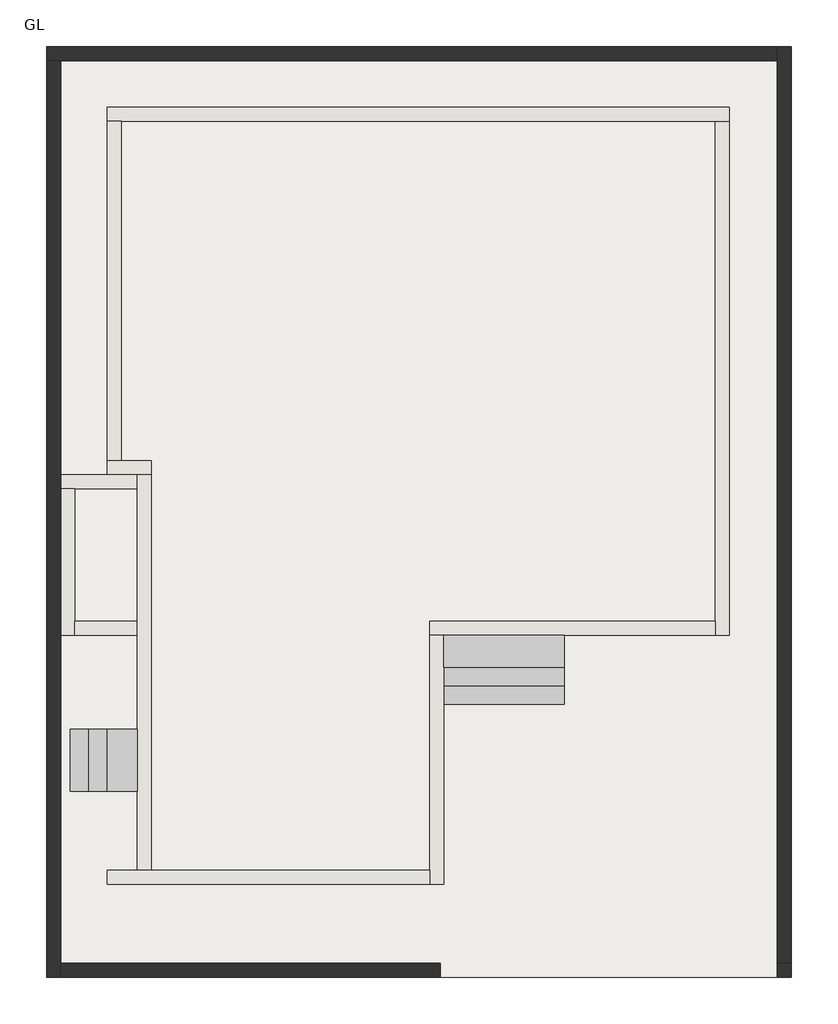
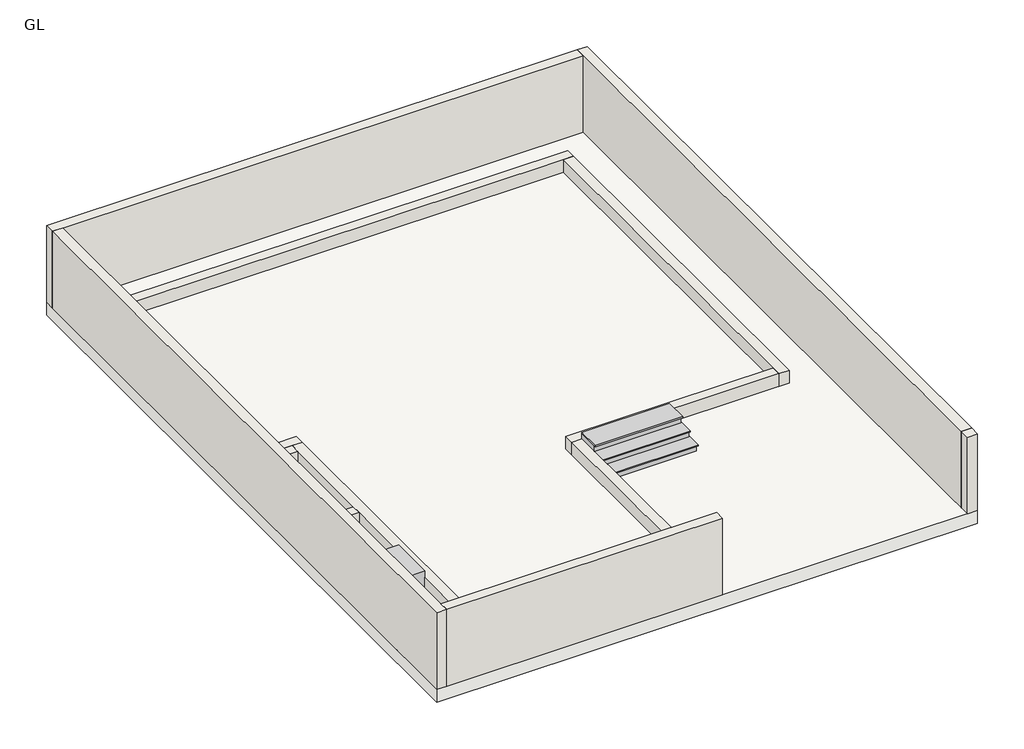
# One storey: 15 walls, 2 proxies, 1 slab.
"""IFC4 building model written with IfcOpenShell, lengths in millimetres."""

from ifc_helpers import new_model, si_unit, frame, origin, place, context, project, spatial, polyline, outline, extrude, faceted_brep, transform, mapped, element, save
from components import generic_models_1_generic_models_1_70b2dbcb, generic_models_2_generic_models_1_31704990

model = new_model("IFC4")

# Units and contexts
model_context = context("Model", 3, world=origin())
ifc_project = project(units=[si_unit("LENGTHUNIT", "METRE", prefix="MILLI")], contexts=[model_context])

# Site, building, storey
site = spatial("IfcSite", under=ifc_project)
building = spatial("IfcBuilding", under=site)
storey = spatial("IfcBuildingStorey", under=building, Name="GL", Elevation=-457.2)

# Proxies
placement = place(None, origin())
generic_models_1_generic_models_1_shape = generic_models_1_generic_models_1_70b2dbcb(model_context)
element("IfcBuildingElementProxy", 1, Name="Generic Models 1 : Generic Models 1", ObjectType="Generic Models 1 : Generic Models 1", at=placement, inside=storey, context=model_context, shape_type="MappedRepresentation", body=[
    mapped(generic_models_1_generic_models_1_shape, transform((0.0, 0.0, 0.0), x_axis=(1.0, 0.0, 0.0), y_axis=(0.0, 1.0, 0.0), z_axis=(0.0, 0.0, 1.0))),
])
generic_models_2_generic_models_1_shape = generic_models_2_generic_models_1_31704990(model_context)
element("IfcBuildingElementProxy", 2, Name="Generic Models 2 : Generic Models 1", ObjectType="Generic Models 2 : Generic Models 1", at=placement, inside=storey, context=model_context, shape_type="MappedRepresentation", body=[
    mapped(generic_models_2_generic_models_1_shape, transform((-17182.3129808, -6192.8854878, 0.0), x_axis=(0.0, -1.0, 0.0), y_axis=(1.0, 0.0, 0.0), z_axis=(0.0, 0.0, 1.0))),
])

# Slab
element("IfcSlab", 3, ObjectType="Generic - 12\"", at=placement, inside=storey, context=model_context, shape_type="SweptSolid", body=[
    extrude(outline(polyline([(-2722.9002526, 13392.6128362), (-2722.9002526, -1847.3871638), (-14917.2815026, -1847.3871638), (-14917.2815026, 13392.6128362), (-2722.9002526, 13392.6128362)])), frame((0.0, 0.0, -762.0), z_axis=(0.0, 0.0, 1.0), x_axis=(1.0, 0.0, 0.0)), (0.0, 0.0, 1.0), 304.8),
])

# Walls
element("IfcWall", 4, ObjectType="10\"", at=placement, inside=storey, context=model_context, shape_type="Brep", body=[
    faceted_brep([(-13924.3002526, 12173.4128362, -457.2), (-13695.7002526, 12173.4128362, -457.2), (-3967.5002526, 12173.4128362, -457.2), (-3738.9002526, 12173.4128362, -457.2), (-3738.9002526, 12173.4128362, -152.4), (-3967.5002526, 12173.4128362, -152.4), (-13695.7002526, 12173.4128362, -152.4), (-13924.3002526, 12173.4128362, -152.4), (-13924.3002526, 12402.0128362, -457.2), (-13924.3002526, 12402.0128362, -152.4), (-3738.9002526, 12402.0128362, -152.4), (-3738.9002526, 12402.0128362, -457.2)], [[[0, 1, 2, 3, 4, 5, 6, 7]], [[8, 9, 10, 11]], [[3, 2, 1, 0, 8, 11]], [[7, 6, 5, 4, 10, 9]], [[0, 7, 9, 8]], [[4, 3, 11, 10]]]),
])
element("IfcWall", 5, ObjectType="10\"", at=placement, inside=storey, context=model_context, shape_type="SweptSolid", body=[
    extrude(outline(polyline([(-13695.7002526, 12173.4128362), (-13695.7002526, 6610.8128362), (-13924.3002526, 6610.8128362), (-13924.3002526, 12173.4128362), (-13695.7002526, 12173.4128362)])), frame((0.0, 0.0, -457.2), z_axis=(0.0, 0.0, 1.0), x_axis=(1.0, 0.0, 0.0)), (0.0, 0.0, 1.0), 304.8),
])
element("IfcWall", 6, ObjectType="10\"", at=placement, inside=storey, context=model_context, shape_type="Brep", body=[
    faceted_brep([(-3967.5002526, 12173.4128362, -457.2), (-3967.5002526, 3981.9127283, -457.2), (-3967.5002526, 3753.3127283, -457.2), (-3967.5002526, 3753.3127283, -152.4), (-3967.5002526, 3981.9127283, -152.4), (-3967.5002526, 12173.4128362, -152.4), (-3738.9002526, 12173.4128362, -457.2), (-3738.9002526, 12173.4128362, -152.4), (-3738.9002526, 3753.3127283, -152.4), (-3738.9002526, 3753.3127283, -457.2)], [[[0, 1, 2, 3, 4, 5]], [[6, 7, 8, 9]], [[2, 1, 0, 6, 9]], [[5, 4, 3, 8, 7]], [[0, 5, 7, 6]], [[3, 2, 9, 8]]]),
])
element("IfcWall", 7, ObjectType="10\"", at=placement, inside=storey, context=model_context, shape_type="Brep", body=[
    faceted_brep([(-3967.5002526, 3981.9127283, -457.2), (-8641.1002526, 3981.9127283, -457.2), (-8641.1002526, 3981.9127283, -152.4), (-3967.5002526, 3981.9127283, -152.4), (-3967.5002526, 3753.3127283, -457.2), (-3967.5002526, 3753.3127283, -152.4), (-8412.5002526, 3753.3127283, -152.4), (-8641.1002526, 3753.3127283, -152.4), (-8641.1002526, 3753.3127283, -457.2), (-8412.5002526, 3753.3127283, -457.2)], [[[0, 1, 2, 3]], [[4, 5, 6, 7, 8, 9]], [[1, 0, 4, 9, 8]], [[3, 2, 7, 6, 5]], [[0, 3, 5, 4]], [[2, 1, 8, 7]]]),
])
element("IfcWall", 8, ObjectType="10\"", at=placement, inside=storey, context=model_context, shape_type="Brep", body=[
    faceted_brep([(-8641.1002526, 3753.3127283, -457.2), (-8641.1002526, -92.4059138, -457.2), (-8641.1002526, -321.0059138, -457.2), (-8641.1002526, -321.0059138, -152.4), (-8641.1002526, -92.4059138, -152.4), (-8641.1002526, 3753.3127283, -152.4), (-8412.5002526, 3753.3127283, -457.2), (-8412.5002526, 3753.3127283, -152.4), (-8412.5002526, -321.0059138, -152.4), (-8412.5002526, -321.0059138, -457.2)], [[[0, 1, 2, 3, 4, 5]], [[6, 7, 8, 9]], [[2, 1, 0, 6, 9]], [[5, 4, 3, 8, 7]], [[0, 5, 7, 6]], [[3, 2, 9, 8]]]),
])
element("IfcWall", 9, ObjectType="10\"", at=placement, inside=storey, context=model_context, shape_type="Brep", body=[
    faceted_brep([(-8641.1002526, -92.4059138, -457.2), (-13200.4002526, -92.4059138, -457.2), (-13429.0002526, -92.4059138, -457.2), (-13925.8877526, -92.4059138, -457.2), (-13925.8877526, -92.4059138, -152.4), (-13429.0002526, -92.4059138, -152.4), (-13200.4002526, -92.4059138, -152.4), (-8641.1002526, -92.4059138, -152.4), (-8641.1002526, -321.0059138, -457.2), (-8641.1002526, -321.0059138, -152.4), (-13925.8877526, -321.0059138, -152.4), (-13925.8877526, -321.0059138, -457.2)], [[[0, 1, 2, 3, 4, 5, 6, 7]], [[8, 9, 10, 11]], [[3, 2, 1, 0, 8, 11]], [[4, 3, 11, 10]], [[7, 6, 5, 4, 10, 9]], [[0, 7, 9, 8]]]),
])
element("IfcWall", 10, ObjectType="10\"", at=placement, inside=storey, context=model_context, shape_type="Brep", body=[
    faceted_brep([(-13200.4002526, -92.4059138, -457.2), (-13200.4002526, 6382.2128362, -457.2), (-13200.4002526, 6382.2128362, -152.4), (-13200.4002526, -92.4059138, -152.4), (-13429.0002526, -92.4059138, -457.2), (-13429.0002526, -92.4059138, -152.4), (-13429.0002526, 3752.3673766, -152.4), (-13429.0002526, 3980.9673766, -152.4), (-13429.0002526, 6153.6128362, -152.4), (-13429.0002526, 6382.2128362, -152.4), (-13429.0002526, 6382.2128362, -457.2), (-13429.0002526, 6153.6128362, -457.2), (-13429.0002526, 3980.9673766, -457.2), (-13429.0002526, 3752.3673766, -457.2)], [[[0, 1, 2, 3]], [[4, 5, 6, 7, 8, 9, 10, 11, 12, 13]], [[1, 0, 4, 13, 12, 11, 10]], [[3, 2, 9, 8, 7, 6, 5]], [[0, 3, 5, 4]], [[2, 1, 10, 9]]]),
])
element("IfcWall", 11, ObjectType="10\"", at=placement, inside=storey, context=model_context, shape_type="Brep", body=[
    faceted_brep([(-13924.3002526, 6382.2128362, -457.2), (-13429.0002526, 6382.2128362, -457.2), (-13200.4002526, 6382.2128362, -457.2), (-13200.4002526, 6382.2128362, -152.4), (-13429.0002526, 6382.2128362, -152.4), (-13924.3002526, 6382.2128362, -152.4), (-13924.3002526, 6610.8128362, -457.2), (-13924.3002526, 6610.8128362, -152.4), (-13695.7002526, 6610.8128362, -152.4), (-13200.4002526, 6610.8128362, -152.4), (-13200.4002526, 6610.8128362, -457.2), (-13695.7002526, 6610.8128362, -457.2)], [[[0, 1, 2, 3, 4, 5]], [[6, 7, 8, 9, 10, 11]], [[2, 1, 0, 6, 11, 10]], [[5, 4, 3, 9, 8, 7]], [[0, 5, 7, 6]], [[3, 2, 10, 9]]]),
])
element("IfcWall", 12, ObjectType="10\"", at=placement, inside=storey, context=model_context, shape_type="Brep", body=[
    faceted_brep([(-14686.3002526, 6153.6128362, -457.2), (-14457.7002526, 6153.6128362, -457.2), (-13429.0002526, 6153.6128362, -457.2), (-13429.0002526, 6153.6128362, -152.4), (-14457.7002526, 6153.6128362, -152.4), (-14686.3002526, 6153.6128362, -152.4), (-14686.3002526, 6382.2128362, -457.2), (-14686.3002526, 6382.2128362, -152.4), (-13429.0002526, 6382.2128362, -152.4), (-13429.0002526, 6382.2128362, -457.2)], [[[0, 1, 2, 3, 4, 5]], [[6, 7, 8, 9]], [[2, 1, 0, 6, 9]], [[5, 4, 3, 8, 7]], [[0, 5, 7, 6]], [[3, 2, 9, 8]]]),
])
element("IfcWall", 13, ObjectType="10\"", at=placement, inside=storey, context=model_context, shape_type="Brep", body=[
    faceted_brep([(-14457.7002526, 3752.3673766, -457.2), (-14457.7002526, 3980.9673766, -457.2), (-14457.7002526, 6153.6128362, -457.2), (-14457.7002526, 6153.6128362, -152.4), (-14457.7002526, 3980.9673766, -152.4), (-14457.7002526, 3752.3673766, -152.4), (-14686.3002526, 3752.3673766, -457.2), (-14686.3002526, 3752.3673766, -152.4), (-14686.3002526, 6153.6128362, -152.4), (-14686.3002526, 6153.6128362, -457.2)], [[[0, 1, 2, 3, 4, 5]], [[6, 7, 8, 9]], [[2, 1, 0, 6, 9]], [[5, 4, 3, 8, 7]], [[3, 2, 9, 8]], [[0, 5, 7, 6]]]),
])
element("IfcWall", 14, ObjectType="10\"", at=placement, inside=storey, context=model_context, shape_type="SweptSolid", body=[
    extrude(outline(polyline([(-14457.7002526, 3980.9673766), (-13429.0002526, 3980.9673766), (-13429.0002526, 3752.3673766), (-14457.7002526, 3752.3673766), (-14457.7002526, 3980.9673766)])), frame((0.0, 0.0, -457.2), z_axis=(0.0, 0.0, 1.0), x_axis=(1.0, 0.0, 0.0)), (0.0, 0.0, 1.0), 304.8),
])
element("IfcWall", 15, ObjectType="10\"", at=placement, inside=storey, context=model_context, shape_type="Brep", body=[
    faceted_brep([(-14917.2815026, 13164.0128362, -457.2), (-14688.6815026, 13164.0128362, -457.2), (-2951.5002526, 13164.0128362, -457.2), (-2951.5002526, 13164.0128362, 1371.6), (-14688.6815026, 13164.0128362, 1371.6), (-14917.2815026, 13164.0128362, 1371.6), (-14917.2815026, 13392.6128362, -457.2), (-14917.2815026, 13392.6128362, 1371.6), (-2951.5002526, 13392.6128362, 1371.6), (-2951.5002526, 13392.6128362, -457.2)], [[[0, 1, 2, 3, 4, 5]], [[6, 7, 8, 9]], [[2, 1, 0, 6, 9]], [[5, 4, 3, 8, 7]], [[0, 5, 7, 6]], [[3, 2, 9, 8]]]),
])
element("IfcWall", 16, ObjectType="10\"", at=placement, inside=storey, context=model_context, shape_type="Brep", body=[
    faceted_brep([(-14688.6815026, -1847.3871638, -457.2), (-14688.6815026, -1618.7871638, -457.2), (-14688.6815026, 13164.0128362, -457.2), (-14688.6815026, 13164.0128362, 1371.6), (-14688.6815026, -1618.7871638, 1371.6), (-14688.6815026, -1847.3871638, 1371.6), (-14917.2815026, -1847.3871638, -457.2), (-14917.2815026, -1847.3871638, 1371.6), (-14917.2815026, 13164.0128362, 1371.6), (-14917.2815026, 13164.0128362, -457.2)], [[[0, 1, 2, 3, 4, 5]], [[6, 7, 8, 9]], [[2, 1, 0, 6, 9]], [[5, 4, 3, 8, 7]], [[0, 5, 7, 6]], [[3, 2, 9, 8]]]),
])
element("IfcWall", 17, ObjectType="10\"", at=placement, inside=storey, context=model_context, shape_type="Brep", body=[
    faceted_brep([(-14688.6815026, -1618.7871638, -457.2), (-14688.6815026, -1618.7871638, 1371.6), (-8473.0253965, -1618.7871638, 1371.6), (-8473.0253965, -1618.7871638, -457.2), (-14688.6815026, -1847.3871638, 1371.6), (-14688.6815026, -1847.3871638, -457.2), (-8473.0253965, -1847.3871638, -457.2), (-8473.0253965, -1847.3871638, 1371.6)], [[[0, 1, 2, 3]], [[4, 5, 6, 7]], [[5, 0, 3, 6]], [[1, 4, 7, 2]], [[1, 0, 5, 4]], [[3, 2, 7, 6]]]),
    faceted_brep([(-2722.9002526, -1618.7871638, 1371.6), (-2722.9002526, -1618.7871638, -457.2), (-2951.5002526, -1618.7871638, -457.2), (-2951.6894507, -1618.7871638, -457.2), (-2951.6894507, -1618.7871638, 1371.6), (-2951.5002526, -1618.7871638, 1371.6), (-2722.9002526, -1847.3871638, -457.2), (-2722.9002526, -1847.3871638, 1371.6), (-2951.6894507, -1847.3871638, 1371.6), (-2951.6894507, -1847.3871638, -457.2)], [[[0, 1, 2, 3, 4, 5]], [[6, 7, 8, 9]], [[1, 6, 9, 3, 2]], [[7, 0, 5, 4, 8]], [[1, 0, 7, 6]], [[4, 3, 9, 8]]]),
])
element("IfcWall", 18, ObjectType="10\"", at=placement, inside=storey, context=model_context, shape_type="Brep", body=[
    faceted_brep([(-2951.5002526, 13392.6128362, -457.2), (-2951.5002526, 13164.0128362, -457.2), (-2951.5002526, -1618.7871638, -457.2), (-2951.5002526, -1618.7871638, 1371.6), (-2951.5002526, 13164.0128362, 1371.6), (-2951.5002526, 13392.6128362, 1371.6), (-2722.9002526, 13392.6128362, -457.2), (-2722.9002526, 13392.6128362, 1371.6), (-2722.9002526, -1618.7871638, 1371.6), (-2722.9002526, -1618.7871638, -457.2)], [[[0, 1, 2, 3, 4, 5]], [[6, 7, 8, 9]], [[2, 1, 0, 6, 9]], [[5, 4, 3, 8, 7]], [[0, 5, 7, 6]], [[3, 2, 9, 8]]]),
])

save(model, "model.ifc")

# Revit data of these elements
# Type "Generic - 12\""
#   Assembly Code = "B1010"
#   Function = 0
#   Layers, outside or top first: 1' - 0" no material (function 1)
# Type "10\""
#   Assembly Code = "B2010"
#   Layers, outside or top first: 0' - 9" "Gypsum Wall Board" (function 1)
# Element 1 (IfcBuildingElementProxy, "Generic Models 1 : Generic Models 1")
#   Phase Created = New Construction
#   Materials on its faces: "BLACK GRANITE"
# Element 2 (IfcBuildingElementProxy, "Generic Models 2 : Generic Models 1")
#   Phase Created = New Construction
# Element 3 (IfcSlab, "Generic - 12\"")
#   Height Offset From Level = 0' - 0"
#   Phase Created = New Construction
#   Materials on its faces: "Default Floor"
# Elements 4, 5, 6, 7, 8, 9, 10, 11, 12, 13, 14 (IfcWall, "10\"")
#   Top Offset = 0' - 0"
#   Base Offset = 0' - 0"
#   Unconnected Height = 1' - 0"
#   wall height = 1' - 0"
#   Phase Created = New Construction
#   Base Constraint = GL
#   Materials on its faces: "Gypsum Wall Board"
# Elements 15, 16, 17, 18 (IfcWall, "10\"")
#   Top Offset = 0' - 0"
#   Base Offset = 0' - 0"
#   Unconnected Height = 6' - 0"
#   wall height = 6' - 0"
#   Phase Created = New Construction
#   Base Constraint = GL
#   Materials on its faces: "Gypsum Wall Board"
# Materials
#   "Gypsum Wall Board": class "Generic", colour RGB 228 228 228, transparency 0, Description = "Gypsum Wall Board", Cost = 0
#   "BLACK GRANITE": class "Generic", colour RGB 42 42 42, transparency 0, Cost = 0
#   "Default Floor": colour RGB 128 128 128, transparency 0, Cost = 0
